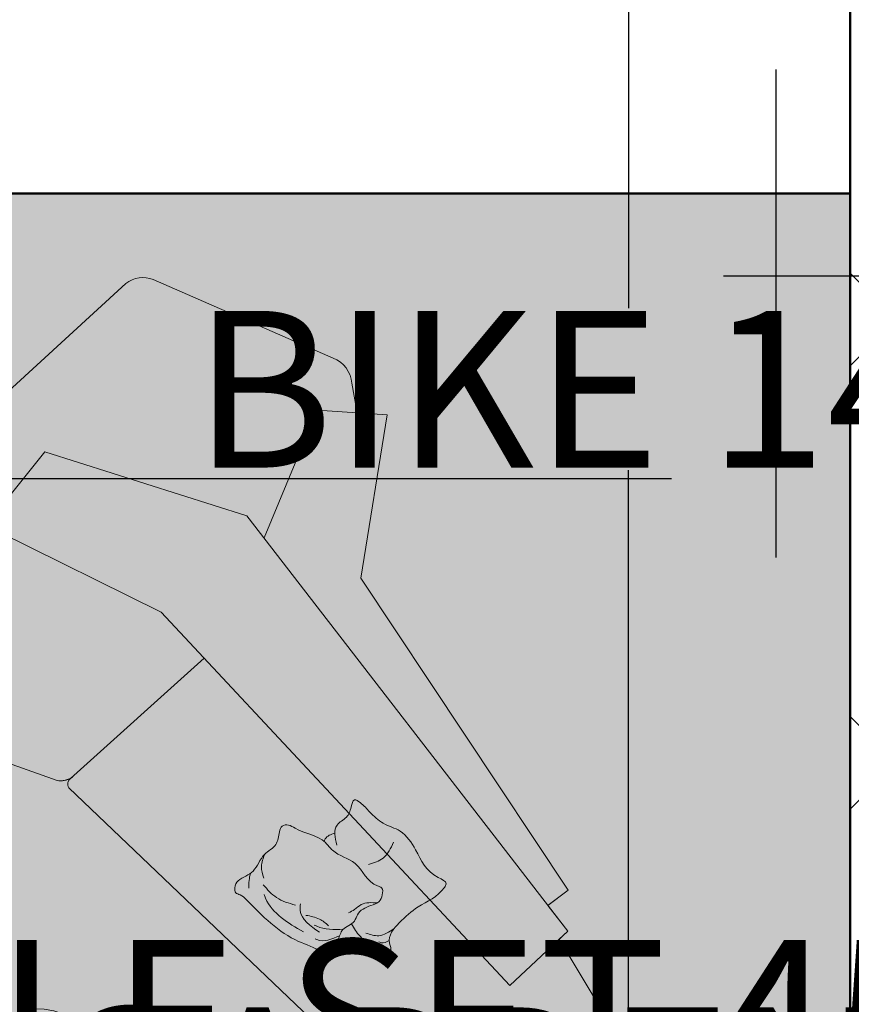
# Model space of a CAD drawing. Units: inches. Extents: x -466983 to 1020, y 324 to 318697.
# Tile 18 of 97: x 782 to 814, y 473 to 511. Entities that reach past the tile are written whole.
import ezdxf

# ---------------------------------------------------------------- set-up
doc = ezdxf.new("R2010")
doc.units = ezdxf.units.IN
doc.header["$MEASUREMENT"] = 0
for name, color, linetype, lineweight in [('A-ANNO-DIMS', 2, 'Continuous', 18), ('A-FLOR-PATT', 252, 'Continuous', 13), ('A-FURN', 8, 'Continuous', 18), ('A-WALL', 7, 'Continuous', 50)]:
    doc.layers.add(name, color=color, linetype=linetype, lineweight=lineweight)
doc.layers.add('K-Hatch', color=7, linetype='Continuous')
doc.styles.get("Standard").update_dxf_attribs({"font": 'arial.ttf'})
doc.dimstyles.get("Standard").update_dxf_attribs({"dimtxt": 6, "dimasz": 4, "dimexe": 3, "dimexo": 3, "dimgap": 0.09, "dimtad": 0, "dimtih": 1, "dimtoh": 1, "dimdec": 1, "dimzin": 0, "dimdsep": 46, "dimlunit": 3, "dimtxsty": 'Standard', "dimcen": 0.09, "dimadec": 0, "dimazin": 0, "dimtfac": 1, "dimtdec": 1, "dimtofl": 0, "dimtmove": 0, "dimatfit": 3, "dimfxl": 1, "dimtolj": 1, "dimtzin": 0, "dimarcsym": 0})

# ---------------------------------------------------------------- blocks, each defined once
blk = doc.blocks.new('CBV_08')
at = {"layer": 'K-Hatch'}
h = blk.add_hatch(color=256, dxfattribs=at)
h.dxf.hatch_style = 1
h.set_gradient(color1=(254, 240, 205), color2=(128, 128, 128), name='INVSPHERICAL')
edge = h.paths.add_edge_path()
edge.add_line((-64.8, 606.5), (-20.8, 613.5))
edge.add_line((-20.8, 613.5), (24.3, 618.7))
edge.add_line((24.3, 618.7), (72.9, 622.4))
edge.add_line((72.9, 622.4), (121.2, 624.4))
edge.add_line((121.2, 624.4), (138, 624.4))
edge.add_spline(control_points=[(138, 624.4), (115.4, 642), (92.5, 659.2), (69.5, 676.1)], knot_values=[4, 4, 4, 4, 4.295361, 4.295361, 4.295361, 4.295361], degree=3, periodic=0)
edge.add_spline(control_points=[(69.5, 676.1), (30.7, 704.6), (-11, 728.2), (-55.3, 747.2)], knot_values=[3, 3, 3, 3, 4, 4, 4, 4], degree=3, periodic=0)
edge.add_spline(control_points=[(-55.3, 747.2), (-74.8, 755.6), (-96, 763.3), (-117, 767)], knot_values=[2, 2, 2, 2, 3, 3, 3, 3], degree=3, periodic=0)
edge.add_spline(control_points=[(-117, 767), (-129.2, 769.1), (-142.6, 773.4), (-154.9, 773.6)], knot_values=[1, 1, 1, 1, 2, 2, 2, 2], degree=3, periodic=0)
edge.add_spline(control_points=[(-154.9, 773.6), (-167.5, 773.8), (-180, 774.1), (-192.6, 774.3)], knot_values=[0, 0, 0, 0, 1, 1, 1, 1], degree=3, periodic=0)
edge.add_spline(control_points=[(-192.6, 774.3), (-216.8, 770.8), (-242.2, 768.1), (-264.6, 757.4)], knot_values=[36, 36, 36, 36, 37, 37, 37, 37], degree=3, periodic=0)
edge.add_spline(control_points=[(-264.6, 757.4), (-290.4, 745.1), (-313.9, 731.3), (-338.2, 716.3)], knot_values=[35, 35, 35, 35, 36, 36, 36, 36], degree=3, periodic=0)
edge.add_spline(control_points=[(-338.2, 716.3), (-348, 710.3), (-356.8, 702.3), (-365.9, 695.4)], knot_values=[34, 34, 34, 34, 35, 35, 35, 35], degree=3, periodic=0)
edge.add_spline(control_points=[(-365.9, 695.4), (-373.7, 689.5), (-381.9, 684), (-389, 677.3)], knot_values=[33, 33, 33, 33, 34, 34, 34, 34], degree=3, periodic=0)
edge.add_spline(control_points=[(-389, 677.3), (-406.7, 660.6), (-425.2, 644.6), (-441, 625.9)], knot_values=[32, 32, 32, 32, 33, 33, 33, 33], degree=3, periodic=0)
edge.add_spline(control_points=[(-441, 625.9), (-457.4, 606.6), (-473.1, 588.1), (-486.9, 566.8)], knot_values=[31, 31, 31, 31, 32, 32, 32, 32], degree=3, periodic=0)
edge.add_spline(control_points=[(-486.9, 566.8), (-500.9, 545.3), (-513.6, 524.6), (-525.3, 501.8)], knot_values=[30, 30, 30, 30, 31, 31, 31, 31], degree=3, periodic=0)
edge.add_spline(control_points=[(-525.3, 501.8), (-537.3, 478.5), (-547, 455.6), (-556.5, 431.1)], knot_values=[29, 29, 29, 29, 30, 30, 30, 30], degree=3, periodic=0)
edge.add_spline(control_points=[(-556.5, 431.1), (-560.1, 422), (-562.6, 413.9), (-564.7, 404.4)], knot_values=[28, 28, 28, 28, 29, 29, 29, 29], degree=3, periodic=0)
edge.add_spline(control_points=[(-564.7, 404.4), (-567.4, 392.4), (-572.8, 378.6), (-573.3, 366.3)], knot_values=[27, 27, 27, 27, 28, 28, 28, 28], degree=3, periodic=0)
edge.add_spline(control_points=[(-573.3, 366.3), (-574.1, 341.5), (-575.3, 317.8), (-572.6, 293.2)], knot_values=[26, 26, 26, 26, 27, 27, 27, 27], degree=3, periodic=0)
edge.add_spline(control_points=[(-572.6, 293.2), (-569.8, 268.3), (-564.7, 244.8), (-559.2, 220.4)], knot_values=[25, 25, 25, 25, 26, 26, 26, 26], degree=3, periodic=0)
edge.add_spline(control_points=[(-559.2, 220.4), (-554.1, 197.5), (-542.3, 175), (-531.2, 154.5)], knot_values=[24, 24, 24, 24, 25, 25, 25, 25], degree=3, periodic=0)
edge.add_spline(control_points=[(-531.2, 154.5), (-519.4, 132.5), (-505, 113.3), (-490.3, 93.1)], knot_values=[23, 23, 23, 23, 24, 24, 24, 24], degree=3, periodic=0)
edge.add_spline(control_points=[(-490.3, 93.1), (-483.4, 83.5), (-474, 75.1), (-466, 66.4)], knot_values=[22, 22, 22, 22, 23, 23, 23, 23], degree=3, periodic=0)
edge.add_spline(control_points=[(-466, 66.4), (-459.7, 59.5), (-453.6, 52.4), (-446.7, 46)], knot_values=[21, 21, 21, 21, 22, 22, 22, 22], degree=3, periodic=0)
edge.add_spline(control_points=[(-446.7, 46), (-428.9, 29.8), (-411.7, 12.8), (-392.8, -2.2)], knot_values=[20, 20, 20, 20, 21, 21, 21, 21], degree=3, periodic=0)
edge.add_spline(control_points=[(-392.8, -2.2), (-354.9, -32.3), (-316.7, -63.5), (-274.7, -87.8)], knot_values=[19, 19, 19, 19, 20, 20, 20, 20], degree=3, periodic=0)
edge.add_spline(control_points=[(-274.7, -87.8), (-235, -110.9), (-195.1, -133.6), (-153.3, -152.9)], knot_values=[18.058389, 18.058389, 18.058389, 18.058389, 19, 19, 19, 19], degree=3, periodic=0)
edge.add_arc((49.9, -261.3), 230.3, 65.0387, 151.9024, ccw=False)
edge.add_arc((-129.3, -568), 584.8, 31.4853, 61.8022, ccw=False)
edge.add_spline(control_points=[(369.5, -262.5), (382.1, -256.3), (394.4, -248.9), (404.8, -240.3)], knot_values=[14, 14, 14, 14, 14.639139, 14.639139, 14.639139, 14.639139], degree=3, periodic=0)
edge.add_spline(control_points=[(404.8, -240.3), (441.3, -209.9), (479.6, -177), (505.1, -136.3)], knot_values=[13, 13, 13, 13, 14, 14, 14, 14], degree=3, periodic=0)
edge.add_spline(control_points=[(505.1, -136.3), (530.8, -95.3), (553.2, -52.4), (563.4, -4.8)], knot_values=[12, 12, 12, 12, 13, 13, 13, 13], degree=3, periodic=0)
edge.add_spline(control_points=[(563.4, -4.8), (565.9, 6.8), (569.9, 18.9), (570.9, 30.6)], knot_values=[11, 11, 11, 11, 12, 12, 12, 12], degree=3, periodic=0)
edge.add_spline(control_points=[(570.9, 30.6), (572, 44.6), (573.1, 58.6), (574.2, 72.5)], knot_values=[10, 10, 10, 10, 11, 11, 11, 11], degree=3, periodic=0)
edge.add_spline(control_points=[(574.2, 72.5), (575.1, 84.1), (571.6, 97.4), (570.3, 109)], knot_values=[9, 9, 9, 9, 10, 10, 10, 10], degree=3, periodic=0)
edge.add_spline(control_points=[(570.3, 109), (569.1, 120.8), (562.9, 133.2), (559.3, 144.5)], knot_values=[8, 8, 8, 8, 9, 9, 9, 9], degree=3, periodic=0)
edge.add_spline(control_points=[(559.3, 144.5), (552.8, 164.6), (542, 184.7), (531.4, 203)], knot_values=[7, 7, 7, 7, 8, 8, 8, 8], degree=3, periodic=0)
edge.add_spline(control_points=[(531.4, 203), (517.9, 226.2), (504.2, 248.2), (488.9, 270.1)], knot_values=[6, 6, 6, 6, 7, 7, 7, 7], degree=3, periodic=0)
edge.add_spline(control_points=[(488.9, 270.1), (469.9, 297.6), (449.2, 323.8), (427.6, 349.1)], knot_values=[5.661323, 5.661323, 5.661323, 5.661323, 6, 6, 6, 6], degree=3, periodic=0)
edge.add_line((427.6, 349.1), (424, 340.6))
edge.add_line((424, 340.6), (412.8, 320.4))
edge.add_line((412.8, 320.4), (399.8, 302.2))
edge.add_line((399.8, 302.2), (384.1, 283.9))
edge.add_line((384.1, 283.9), (364.2, 265.4))
edge.add_line((364.2, 265.4), (338.9, 246.4))
edge.add_line((338.9, 246.4), (310.9, 228.8))
edge.add_line((310.9, 228.8), (283, 214))
edge.add_line((283, 214), (254.8, 200.7))
edge.add_line((254.8, 200.7), (225.6, 187.8))
edge.add_line((225.6, 187.8), (191.9, 174.7))
edge.add_line((191.9, 174.7), (149.8, 160.6))
edge.add_line((149.8, 160.6), (105.2, 147.1))
edge.add_line((105.2, 147.1), (63.8, 135.5))
edge.add_line((63.8, 135.5), (25.5, 126.4))
edge.add_line((25.5, 126.4), (-10.1, 120.3))
edge.add_line((-10.1, 120.3), (-42.7, 117))
edge.add_line((-42.7, 117), (-72.3, 116.4))
edge.add_line((-72.3, 116.4), (-101, 119.4))
edge.add_line((-101, 119.4), (-131.2, 126.4))
edge.add_line((-131.2, 126.4), (-161, 137.6))
edge.add_line((-161, 137.6), (-188.5, 153.1))
edge.add_line((-188.5, 153.1), (-212.6, 173.8))
edge.add_line((-212.6, 173.8), (-232.4, 200.6))
edge.add_line((-232.4, 200.6), (-247.5, 230.4))
edge.add_line((-247.5, 230.4), (-258, 260.2))
edge.add_line((-258, 260.2), (-265.5, 290.4))
edge.add_line((-265.5, 290.4), (-271.7, 321.1))
edge.add_line((-271.7, 321.1), (-275.7, 353.5))
edge.add_line((-275.7, 353.5), (-276.1, 388.5))
edge.add_line((-276.1, 388.5), (-273.5, 421.6))
edge.add_line((-273.5, 421.6), (-268.6, 448.2))
edge.add_line((-268.6, 448.2), (-261.6, 470.9))
edge.add_line((-261.6, 470.9), (-253.2, 492.6))
edge.add_line((-253.2, 492.6), (-243.7, 512.2))
edge.add_line((-243.7, 512.2), (-233.7, 528.6))
edge.add_line((-233.7, 528.6), (-222.4, 543.2))
edge.add_line((-222.4, 543.2), (-208.8, 557))
edge.add_line((-208.8, 557), (-193, 569.1))
edge.add_line((-193, 569.1), (-174.9, 578.6))
edge.add_line((-174.9, 578.6), (-149, 587.3))
edge.add_line((-149, 587.3), (-109.9, 597.2))
edge.add_line((-109.9, 597.2), (-64.8, 606.5))
edge = h.paths.add_edge_path()
edge.add_spline(control_points=[(370.8, -764.2), (495.7, -715.3), (556.2, -553.3), (490.4, -435.8)], knot_values=[8, 8, 8, 8, 9, 9, 9, 9], degree=3, periodic=0)
edge.add_spline(control_points=[(490.4, -435.8), (456.6, -375.3), (415.1, -316.6), (369.5, -262.5)], knot_values=[7.311196, 7.311196, 7.311196, 7.311196, 8, 8, 8, 8], degree=3, periodic=0)
edge.add_spline(control_points=[(369.5, -262.5), (362.3, -266), (355, -269.1), (347.9, -271.7)], knot_values=[14.639139, 14.639139, 14.639139, 14.639139, 15, 15, 15, 15], degree=3, periodic=0)
edge.add_spline(control_points=[(347.9, -271.7), (326, -279.9), (303.4, -287.9), (279.6, -286.9)], knot_values=[15, 15, 15, 15, 16, 16, 16, 16], degree=3, periodic=0)
edge.add_spline(control_points=[(279.6, -286.9), (229.3, -284.8), (181, -274.1), (132.3, -261.7)], knot_values=[16, 16, 16, 16, 17, 17, 17, 17], degree=3, periodic=0)
edge.add_spline(control_points=[(132.3, -261.7), (36, -237.2), (-55, -196.9), (-145.5, -156.4)], knot_values=[17, 17, 17, 17, 18, 18, 18, 18], degree=3, periodic=0)
edge.add_spline(control_points=[(-145.5, -156.4), (-148.1, -155.2), (-150.7, -154.1), (-153.3, -152.9)], knot_values=[18, 18, 18, 18, 18.058389, 18.058389, 18.058389, 18.058389], degree=3, periodic=0)
edge.add_spline(control_points=[(-274.7, -87.8), (-235, -110.9), (-195.1, -133.6), (-153.3, -152.9)], knot_values=[18.058389, 18.058389, 18.058389, 18.058389, 19, 19, 19, 19], degree=3, periodic=0)
edge.add_spline(control_points=[(-153.3, -152.9), (-166, -171.6), (-175.5, -191.9), (-179.2, -212.7)], knot_values=[4, 4, 4, 4, 4.452929, 4.452929, 4.452929, 4.452929], degree=3, periodic=0)
edge.add_spline(control_points=[(-179.2, -212.7), (-197.4, -316.3), (-177.2, -425), (-133.8, -520.2)], knot_values=[3, 3, 3, 3, 4, 4, 4, 4], degree=3, periodic=0)
edge.add_spline(control_points=[(-133.8, -520.2), (-113.8, -564.2), (-89.7, -609.8), (-55.6, -644.7)], knot_values=[2, 2, 2, 2, 3, 3, 3, 3], degree=3, periodic=0)
edge.add_spline(control_points=[(-55.6, -644.7), (-21, -680), (24.1, -705.5), (69.8, -723.3)], knot_values=[1, 1, 1, 1, 2, 2, 2, 2], degree=3, periodic=0)
edge.add_spline(control_points=[(69.8, -723.3), (165.7, -760.7), (268.3, -790.7), (370.8, -764.2)], knot_values=[0, 0, 0, 0, 1, 1, 1, 1], degree=3, periodic=0)
h = blk.add_hatch(color=256, dxfattribs=at)
h.dxf.hatch_style = 1
h.set_gradient(color1=(237, 238, 153), color2=(128, 128, 128), name='INVSPHERICAL')
h.paths.add_polyline_path([(138, 624.4), (121.2, 624.4), (72.9, 622.4), (24.3, 618.7), (-20.8, 613.5), (-64.8, 606.5), (-109.9, 597.2), (-149, 587.3), (-174.9, 578.6), (-193, 569.1), (-208.8, 557), (-222.4, 543.2), (-233.7, 528.6), (-243.7, 512.2), (-253.2, 492.6), (-261.6, 470.9), (-268.6, 448.2), (-273.5, 421.6), (-276.1, 388.5), (-275.7, 353.5), (-271.7, 321.1), (-265.5, 290.4), (-258, 260.2), (-247.5, 230.4), (-232.4, 200.6), (-212.6, 173.8), (-188.5, 153.1), (-161, 137.6), (-131.2, 126.4), (-101, 119.4), (-72.3, 116.4), (-42.7, 117), (-10.1, 120.3), (25.5, 126.4), (63.8, 135.5), (105.2, 147.1), (149.8, 160.6), (191.9, 174.7), (225.6, 187.8), (254.8, 200.7), (283, 214), (310.9, 228.8), (338.9, 246.4), (364.2, 265.4), (384.1, 283.9), (399.8, 302.2), (412.8, 320.4), (424, 340.6), (427.6, 349.1, 0.092765)])
h.paths.add_polyline_path([(388.8, 558), (367.1, 577.3), (341.1, 593.1), (309.7, 604.8), (275.6, 613.2), (241.4, 619.1), (205.2, 622.8), (165.2, 624.5), (138, 624.4, -0.092765), (427.6, 349.1), (434.3, 364.7), (441.6, 390.8), (443.8, 416.8), (441.1, 445), (433.5, 477.6), (421.8, 509.5), (406.9, 535.9)])
edge = h.paths.add_edge_path()
edge.add_arc((49.9, -261.3), 230.3, 65.0387, 151.9024)
edge.add_spline(control_points=[(-153.3, -152.9), (-150.7, -154.1), (-148.1, -155.2), (-145.5, -156.4)], knot_values=[18, 18, 18, 18, 18.058389, 18.058389, 18.058389, 18.058389], degree=3, periodic=0)
edge.add_spline(control_points=[(-145.5, -156.4), (-55, -196.9), (36, -237.2), (132.3, -261.7)], knot_values=[17, 17, 17, 17, 18, 18, 18, 18], degree=3, periodic=0)
edge.add_spline(control_points=[(132.3, -261.7), (181, -274.1), (229.3, -284.8), (279.6, -286.9)], knot_values=[16, 16, 16, 16, 17, 17, 17, 17], degree=3, periodic=0)
edge.add_spline(control_points=[(279.6, -286.9), (303.4, -287.9), (326, -279.9), (347.9, -271.7)], knot_values=[15, 15, 15, 15, 16, 16, 16, 16], degree=3, periodic=0)
edge.add_spline(control_points=[(347.9, -271.7), (355, -269.1), (362.3, -266), (369.5, -262.5)], knot_values=[14.639139, 14.639139, 14.639139, 14.639139, 15, 15, 15, 15], degree=3, periodic=0)
edge.add_arc((-129.3, -568), 584.8, 31.4853, 61.8022)
edge = h.paths.add_edge_path()
edge.add_spline(control_points=[(490.4, -435.8), (456.6, -375.3), (415.1, -316.6), (369.5, -262.5)], knot_values=[7.311196, 7.311196, 7.311196, 7.311196, 8, 8, 8, 8], degree=3, periodic=0)
edge.add_spline(control_points=[(369.5, -262.5), (362.3, -266), (355, -269.1), (347.9, -271.7)], knot_values=[14.639139, 14.639139, 14.639139, 14.639139, 15, 15, 15, 15], degree=3, periodic=0)
edge.add_spline(control_points=[(347.9, -271.7), (326, -279.9), (303.4, -287.9), (279.6, -286.9)], knot_values=[15, 15, 15, 15, 16, 16, 16, 16], degree=3, periodic=0)
edge.add_spline(control_points=[(279.6, -286.9), (229.3, -284.8), (181, -274.1), (132.3, -261.7)], knot_values=[16, 16, 16, 16, 17, 17, 17, 17], degree=3, periodic=0)
edge.add_spline(control_points=[(132.3, -261.7), (36, -237.2), (-55, -196.9), (-145.5, -156.4)], knot_values=[17, 17, 17, 17, 18, 18, 18, 18], degree=3, periodic=0)
edge.add_spline(control_points=[(-145.5, -156.4), (-148.1, -155.2), (-150.7, -154.1), (-153.3, -152.9)], knot_values=[18, 18, 18, 18, 18.058389, 18.058389, 18.058389, 18.058389], degree=3, periodic=0)
edge.add_spline(control_points=[(-274.7, -87.8), (-235, -110.9), (-195.1, -133.6), (-153.3, -152.9)], knot_values=[18.058389, 18.058389, 18.058389, 18.058389, 19, 19, 19, 19], degree=3, periodic=0)
edge.add_spline(control_points=[(-153.3, -152.9), (-166, -171.6), (-175.5, -191.9), (-179.2, -212.7)], knot_values=[4, 4, 4, 4, 4.452929, 4.452929, 4.452929, 4.452929], degree=3, periodic=0)
edge.add_spline(control_points=[(-179.2, -212.7), (-197.4, -316.3), (-177.2, -425), (-133.8, -520.2)], knot_values=[3, 3, 3, 3, 4, 4, 4, 4], degree=3, periodic=0)
edge.add_spline(control_points=[(-133.8, -520.2), (-113.8, -564.2), (-89.7, -609.8), (-55.6, -644.7)], knot_values=[2, 2, 2, 2, 3, 3, 3, 3], degree=3, periodic=0)
edge.add_spline(control_points=[(-55.6, -644.7), (-21, -680), (24.1, -705.5), (69.8, -723.3)], knot_values=[1, 1, 1, 1, 2, 2, 2, 2], degree=3, periodic=0)
edge.add_spline(control_points=[(69.8, -723.3), (165.7, -760.7), (268.3, -790.7), (370.8, -764.2)], knot_values=[0, 0, 0, 0, 1, 1, 1, 1], degree=3, periodic=0)
edge.add_spline(control_points=[(370.8, -764.2), (495.7, -715.3), (556.2, -553.3), (490.4, -435.8)], knot_values=[8, 8, 8, 8, 9, 9, 9, 9], degree=3, periodic=0)
for points in [[(24.3, 618.7), (-20.8, 613.5)], [(72.9, 622.4), (24.3, 618.7)], [(121.2, 624.4), (72.9, 622.4)], [(121.2, 624.4), (72.9, 622.4)], [(165.2, 624.5), (121.2, 624.4)], [(205.2, 622.8), (165.2, 624.5)], [(241.4, 619.1), (205.2, 622.8)], [(275.6, 613.2), (241.4, 619.1)], [(-149, 587.3), (-174.9, 578.6)], [(-109.9, 597.2), (-149, 587.3)], [(-64.8, 606.5), (-109.9, 597.2)], [(-20.8, 613.5), (-64.8, 606.5)], [(309.7, 604.8), (275.6, 613.2)], [(341.1, 593.1), (309.7, 604.8)], [(367.1, 577.3), (341.1, 593.1)], [(-208.8, 557), (-222.4, 543.2)], [(-193, 569.1), (-208.8, 557)], [(-174.9, 578.6), (-193, 569.1)], [(388.8, 558), (367.1, 577.3)], [(406.9, 535.9), (388.8, 558)], [(-233.7, 528.6), (-243.7, 512.2)], [(-222.4, 543.2), (-233.7, 528.6)], [(421.8, 509.5), (406.9, 535.9)], [(-253.2, 492.6), (-261.6, 470.9)], [(-243.7, 512.2), (-253.2, 492.6)], [(433.5, 477.6), (421.8, 509.5)], [(-268.6, 448.2), (-273.5, 421.6)], [(-261.6, 470.9), (-268.6, 448.2)], [(441.1, 445), (433.5, 477.6)], [(-273.5, 421.6), (-276.1, 388.5)], [(443.8, 416.8), (441.1, 445)], [(441.6, 390.8), (443.8, 416.8)], [(-276.1, 388.5), (-275.7, 353.5)], [(434.3, 364.7), (441.6, 390.8)], [(-275.7, 353.5), (-271.7, 321.1)], [(424, 340.6), (434.3, 364.7)], [(-271.7, 321.1), (-265.5, 290.4)], [(399.8, 302.2), (412.8, 320.4)], [(412.8, 320.4), (424, 340.6)], [(-265.5, 290.4), (-258, 260.2)], [(364.2, 265.4), (384.1, 283.9)], [(384.1, 283.9), (399.8, 302.2)], [(-258, 260.2), (-247.5, 230.4)], [(310.9, 228.8), (338.9, 246.4)], [(338.9, 246.4), (364.2, 265.4)], [(-247.5, 230.4), (-232.4, 200.6)], [(254.8, 200.7), (283, 214)], [(254.8, 200.7), (283, 214)], [(283, 214), (310.9, 228.8)], [(-232.4, 200.6), (-212.6, 173.8)], [(-212.6, 173.8), (-188.5, 153.1)], [(149.8, 160.6), (191.9, 174.7)], [(149.8, 160.6), (191.9, 174.7)], [(191.9, 174.7), (225.6, 187.8)], [(225.6, 187.8), (254.8, 200.7)], [(227.5, 188.7), (226.1, 188.1)], [(-188.5, 153.1), (-161, 137.6)], [(-161, 137.6), (-131.2, 126.4)], [(63.8, 135.5), (105.2, 147.1)], [(105.2, 147.1), (149.8, 160.6)], [(-131.2, 126.4), (-101, 119.4)], [(-101, 119.4), (-72.3, 116.4)], [(-72.3, 116.4), (-42.7, 117)], [(-42.7, 117), (-10.1, 120.3)], [(-10.1, 120.3), (25.5, 126.4)], [(25.5, 126.4), (63.8, 135.5)]]:
    blk.add_lwpolyline(points)
at = {"ltscale": 150}
for centre, radius, start, end in [((-452.8, -286.9), 1086.1, 35.8442, 57.0436), ((49.9, -261.3), 230.3, 65.0387, 151.9024), ((-129.3, -568), 584.8, 31.4853, 61.8022)]:
    blk.add_arc(centre, radius, start, end, dxfattribs=at)
for points, knots in [([(427.6, 349.1), (449.2, 323.8), (469.9, 297.6), (488.9, 270.1), (504.2, 248.2), (517.9, 226.2), (531.4, 203), (542, 184.7), (552.8, 164.6), (559.3, 144.5), (562.9, 133.2), (569.1, 120.8), (570.3, 109), (571.6, 97.4), (575.1, 84.1), (574.2, 72.5), (573.1, 58.6), (572, 44.6), (570.9, 30.6), (569.9, 18.9), (565.9, 6.8), (563.4, -4.8), (553.2, -52.4), (530.8, -95.3), (505.1, -136.3), (479.6, -177), (441.3, -209.9), (404.8, -240.3), (388.6, -253.7), (367.6, -264.4), (347.9, -271.7), (326, -279.9), (303.4, -287.9), (279.6, -286.9), (229.3, -284.8), (181, -274.1), (132.3, -261.7), (36, -237.2), (-55, -196.9), (-145.5, -156.4), (-190.2, -136.4), (-232.5, -112.4), (-274.7, -87.8), (-316.7, -63.5), (-354.9, -32.3), (-392.8, -2.2), (-411.7, 12.8), (-428.9, 29.8), (-446.7, 46), (-453.6, 52.4), (-459.7, 59.5), (-466, 66.4), (-474, 75.1), (-483.4, 83.5), (-490.3, 93.1), (-505, 113.3), (-519.4, 132.5), (-531.2, 154.5), (-542.3, 175), (-554.1, 197.5), (-559.2, 220.4), (-564.7, 244.8), (-569.8, 268.3), (-572.6, 293.2), (-575.3, 317.8), (-574.1, 341.5), (-573.3, 366.3), (-572.8, 378.6), (-567.4, 392.4), (-564.7, 404.4), (-562.6, 413.9), (-560.1, 422), (-556.5, 431.1), (-547, 455.6), (-537.3, 478.5), (-525.3, 501.8), (-513.6, 524.6), (-500.9, 545.3), (-486.9, 566.8), (-473.1, 588.1), (-457.4, 606.6), (-441, 625.9), (-425.2, 644.6), (-406.7, 660.6), (-389, 677.3), (-381.9, 684), (-373.7, 689.5), (-365.9, 695.4), (-356.8, 702.3), (-348, 710.3), (-338.2, 716.3), (-313.9, 731.3), (-290.4, 745.1), (-264.6, 757.4), (-242.2, 768.1), (-216.8, 770.8), (-192.6, 774.3)], [5.661323, 5.661323, 5.661323, 5.661323, 6, 6, 6, 7, 7, 7, 8, 8, 8, 9, 9, 9, 10, 10, 10, 11, 11, 11, 12, 12, 12, 13, 13, 13, 14, 14, 14, 15, 15, 15, 16, 16, 16, 17, 17, 17, 18, 18, 18, 19, 19, 19, 20, 20, 20, 21, 21, 21, 22, 22, 22, 23, 23, 23, 24, 24, 24, 25, 25, 25, 26, 26, 26, 27, 27, 27, 28, 28, 28, 29, 29, 29, 30, 30, 30, 31, 31, 31, 32, 32, 32, 33, 33, 33, 34, 34, 34, 35, 35, 35, 36, 36, 36, 37, 37, 37, 37]), ([(-192.6, 774.3), (-180, 774.1), (-167.5, 773.8), (-154.9, 773.6), (-142.6, 773.4), (-129.2, 769.1), (-117, 767), (-96, 763.3), (-74.8, 755.6), (-55.3, 747.2), (-11, 728.2), (30.7, 704.6), (69.5, 676.1), (92.5, 659.2), (115.4, 642), (138, 624.4)], [0, 0, 0, 0, 1, 1, 1, 2, 2, 2, 3, 3, 3, 4, 4, 4, 4.295361, 4.295361, 4.295361, 4.295361]), ([(370.8, -764.2), (268.3, -790.7), (165.7, -760.7), (69.8, -723.3), (24.1, -705.5), (-21, -680), (-55.6, -644.7), (-89.7, -609.8), (-113.8, -564.2), (-133.8, -520.2), (-177.2, -425), (-197.4, -316.3), (-179.2, -212.7), (-175.5, -191.9), (-166, -171.6), (-153.3, -152.9)], [0, 0, 0, 0, 1, 1, 1, 2, 2, 2, 3, 3, 3, 4, 4, 4, 4.452929, 4.452929, 4.452929, 4.452929]), ([(369.5, -262.5), (415.1, -316.6), (456.6, -375.3), (490.4, -435.8), (556.2, -553.3), (495.7, -715.3), (370.8, -764.2)], [7.311196, 7.311196, 7.311196, 7.311196, 8, 8, 8, 9, 9, 9, 9])]:
    blk.add_open_spline(points, degree=3, knots=knots)
blk = doc.blocks.new('CBV_05')
at = {"layer": 'K-Hatch'}
h = blk.add_hatch(color=256, dxfattribs=at)
h.dxf.hatch_style = 1
h.paths.add_polyline_path([(614, 437), (1251.4, 62.5), (1198.3, -263.2), (564.8, -9.8), (344.4, -5.5), (343.7, -629.7, 0.159768), (369.9, -672.6), (1020.5, -1025.6, 0.317347), (1135.5, -1017.7), (1739.5, -492.7, 0.378101), (1761.2, -362.2), (1507.4, -70.4, -0.119239), (1492.6, -25.8), (1499.5, 665.1, 0.256804), (1446.2, 745.4), (822.7, 1028.7, 0.297137), (714, 1018.3), (625, 963.6), (549.5, 1037.1), (186.8, 587.5), (-1106.2, 397.7), (-1098.6, 311.5), (-1098.4, 310.2)])
h.paths.add_polyline_path([(344.4, -5.5), (-1216.9, 24.6), (-1212.3, 260), (-1718.1, 162.7, 0.51466), (-1765.1, 50), (-1478.1, -479.5, 0.244482), (-1398.8, -526.6), (323.6, -658.2, 0.453292), (343.1, -629.8, 0.006511), (343.7, -631.8)])
h = blk.add_hatch(color=256, dxfattribs=at)
h.dxf.hatch_style = 1
h.paths.add_polyline_path([(614, 437), (-1211.5, 301.9), (-1212.3, 260), (-1216.9, 24.6), (564.8, -9.8), (1198.3, -263.2), (1251.4, 62.5)])
for p, q in [((186.8, 587.5), (549.5, 1037.1)), ((725.2, 866.1), (549.5, 1037.1)), ((517.5, 431), (725.2, 866.1)), ((-1106.2, 397.7), (186.8, 587.5)), ((-1211.5, 301.9), (614, 437)), ((614, 437), (1251.4, 62.5)), ((-1106.2, 397.7), (-1098.6, 311.5)), ((-1211.5, 301.9), (-1216.9, 24.6)), ((1251.4, 62.5), (1198.3, -263.2)), ((-1216.9, 24.6), (564.8, -9.8)), ((564.8, -9.8), (1198.3, -263.2))]:
    blk.add_line(p, q)
blk.add_lwpolyline([(1761.2, -362.2, -0.378101), (1739.5, -492.7), (1135.5, -1017.7, -0.317347), (1020.5, -1025.6), (369.9, -672.6, -0.159481), (343.2, -630.1, -0.449095), (323.6, -658.2), (-1398.8, -526.6, -0.244482), (-1478.1, -479.5), (-1765.1, 50, -0.51466), (-1718.1, 162.7), (-1212.3, 260), (-1211.5, 301.9), (-1098.4, 310.2), (-1106.2, 397.7), (186.8, 587.5), (549.5, 1037.1), (625, 963.6), (714, 1018.3, -0.297137), (822.7, 1028.7), (1446.2, 745.4, -0.256804), (1499.5, 665.1), (1492.6, -25.8, 0.119239), (1507.4, -70.4)], format="xyb", close=True)
for points in [[(369.9, -672.6), (1020.5, -1025.6, 0.317347), (1135.5, -1017.7), (1739.5, -492.7, 0.378101), (1761.2, -362.2), (1507.4, -70.4, -0.119239), (1492.6, -25.8), (1499.5, 665.1, 0.256804), (1446.2, 745.4), (822.7, 1028.7, 0.297137), (714, 1018.3), (625, 963.6)], [(-1212.3, 260), (-1718.1, 162.7, 0.51466), (-1765.1, 50), (-1478.1, -479.5, 0.244482), (-1398.8, -526.6), (323.6, -658.2)]]:
    blk.add_lwpolyline(points, format="xyb")
blk.add_lwpolyline([(344.4, -5.5), (343.7, -632.6)])
for centre, radius, start, end in [((320.9, -635.5), 22.9, 276.7908, 7.9615), ((422.2, -611.1), 80.7, 188.9571, 229.6497)]:
    blk.add_arc(centre, radius, start, end)
blk = doc.blocks.new('CBV_02')
for points, knots in [([(-91.4, -131.3), (-106.3, -141.3), (-144.4, -166.7), (-198.1, -169.3), (-239.8, -177.4), (-263.2, -156.4), (-220.4, -122.4), (-241.1, -51.6), (-276.5, 31.5), (-327.5, 83.5), (-334.1, 145.3), (-254.2, 139), (-199.8, 191.5), (-115.5, 242.2), (-44.1, 228.2), (13.9, 247.4), (48.9, 263.5), (90.2, 270.4), (80.3, 230.8), (77.5, 197.5), (114.6, 151.6), (88, 117.5), (71.5, 96.3)], [0, 0, 0, 0, 52.878976, 135.54457, 156.895053, 178.454765, 205.017242, 283.653969, 369.581717, 483.880697, 497.901213, 533.111935, 657.57549, 742.691795, 807.096717, 868.633311, 916.15584, 937.624163, 964.928306, 1003.93421, 1046.712597, 1116.246585, 1116.246585, 1116.246585, 1116.246585]), ([(-103.4, 189.4), (-103.5, 166.1), (-103.8, 123.2), (-72.3, 94.8), (-58, 81.8)], [0, 0, 0, 0, 66.320843, 121.78475, 121.78475, 121.78475, 121.78475]), ([(95.2, 131.1), (105.5, 121.2), (118.3, 108.9), (117.4, 92.3), (117.3, 89.1)], [0, 0, 0, 0, 39.264535, 48.815694, 48.815694, 48.815694, 48.815694]), ([(-146.1, 6), (-148.1, -3), (-149.3, -22.5), (-119, -49.5), (-92.3, -81.4), (-102.2, -127.6), (-64.2, -156.5), (-75.8, -196.4), (-68.5, -226.7), (-89.3, -248.7), (-66.3, -271), (-19, -258.2), (97, -276), (211.6, -235.3), (298.4, -201.8), (321.3, -207.8), (333.3, -187), (332.8, -160.3), (312.2, -137.2), (287.8, -99.3), (296.8, -44.1), (256.4, 5), (270.7, 44.3), (276.3, 77.1), (252.3, 90.7), (198.4, 81.4), (134.7, 104), (61.7, 61.2), (-24.3, 81.7), (-82.8, 19.8), (-138, 31.1), (-144, 15.2), (-146.1, 6)], [0, 0, 0, 0, 24.616915, 57.389552, 114.237533, 138.455284, 189.005997, 228.810774, 251.953092, 279.847444, 297.942972, 329.329631, 417.096019, 649.5591, 678.18061, 694.45516, 711.884356, 739.183211, 771.087794, 801.279315, 871.941271, 924.495086, 970.994857, 992.485443, 1014.330787, 1039.800329, 1156.628447, 1193.646246, 1284.736416, 1395.218734, 1410.912041, 1436.038203, 1436.038203, 1436.038203, 1436.038203]), ([(-142.3, -26.5), (-123.8, -33.7), (-95.7, -44.8), (-82, -80.3), (-71.1, -94.3), (-66.1, -100.7)], [0, 0, 0, 0, 56.119763, 85.047758, 109.497008, 109.497008, 109.497008, 109.497008]), ([(285.1, -38.6), (284.4, -54.2), (283, -84.1), (262.6, -105.9), (252.9, -116.4)], [0, 0, 0, 0, 45.245577, 86.676748, 86.676748, 86.676748, 86.676748]), ([(-233.2, -82.9), (-222.4, -100.8), (-203.2, -132.7), (-166.7, -136.8), (-150.7, -138.6)], [0, 0, 0, 0, 58.76228, 104.640212, 104.640212, 104.640212, 104.640212]), ([(-235.6, -127), (-229, -136.1), (-220.7, -147.8), (-207.6, -146.9), (-204.8, -146.7)], [0, 0, 0, 0, 30.082797, 38.252376, 38.252376, 38.252376, 38.252376]), ([(-73.5, -160.3), (-44.8, -174.7), (-13.3, -190.5), (21, -190), (24.2, -189.9)], [0, 0, 0, 0, 92.944368, 102.453901, 102.453901, 102.453901, 102.453901]), ([(-22.2, -170.9), (-9.3, -167.3), (19.5, -159.1), (48.5, -167.1), (64.6, -171.5)], [0, 0, 0, 0, 39.396451, 88.251181, 88.251181, 88.251181, 88.251181]), ([(-2.6, -204.8), (35.3, -198.3), (82, -190.4), (96.8, -150.5), (99.6, -143)], [0, 0, 0, 0, 101.132145, 124.532908, 124.532908, 124.532908, 124.532908]), ([(47.9, -227.8), (110.7, -221.9), (178.7, -215.5), (224.5, -170.7), (228, -167.3)], [0, 0, 0, 0, 176.788032, 191.44385, 191.44385, 191.44385, 191.44385]), ([(244.8, -137.9), (224.6, -146.9), (182.5, -165.9), (136.8, -158.5), (112.9, -154.6)], [0, 0, 0, 0, 64.853922, 135.586683, 135.586683, 135.586683, 135.586683]), ([(-72.1, -185.7), (-52.1, -208.3), (-30.7, -232.6), (-1.5, -232), (0.5, -232)], [0, 0, 0, 0, 81.161444, 87.060878, 87.060878, 87.060878, 87.060878])]:
    blk.add_open_spline(points, degree=3, knots=knots)
blk.add_open_spline([(285.5, -170.2), (292.7, -153.9), (299.9, -137.5), (302.1, -120.4)], degree=3)
blk = doc.blocks.new('Garden Sofa')
at = {"xscale": -0.0109740885734132, "yscale": 0.0109740885734132, "zscale": 0.0109740885734132}
for name, p, rotation in [('CBV_05', (2464.355, 846.083), 311.9356943688126), ('CBV_02', (2467.122, 840.412), 334.8587275215129), ('CBV_08', (2451.373, 829.781), 280.5267845499334)]:
    blk.add_blockref(name, p, dxfattribs=dict(at, rotation=rotation))
blk = doc.blocks.new('*D70')
at = {"layer": 'A-ANNO-DIMS', "color": 0, "lineweight": -2, "transparency": 16777216}
for p, q in [((689.806, 508.686), (689.806, 490.005)), ((810.968, 508.686), (810.968, 490.005)), ((693.806, 493.005), (744.53, 493.005)), ((806.968, 493.005), (756.244, 493.005))]:
    blk.add_line(p, q, dxfattribs=at)
at = {"layer": 'A-ANNO-DIMS', "color": 0, "transparency": 16777216}
for points in [[(693.806, 493.671), (693.806, 492.338), (689.806, 493.005)], [(806.968, 493.671), (806.968, 492.338), (810.968, 493.005)]]:
    blk.add_solid(points, dxfattribs=at)
at = {"layer": 'Defpoints', "color": 0, "transparency": 16777216}
for p in [(689.806, 511.686), (810.968, 511.686), (810.968, 493.005)]:
    blk.add_point(p, dxfattribs=at)
at = {"layer": 'A-ANNO-DIMS', "color": 0, "transparency": 16777216, "insert": (750.387, 493.005), "char_height": 6, "attachment_point": 5}
blk.add_mtext('\\A1;121', dxfattribs=at)
blk = doc.blocks.new('*D93')
at = {"layer": 'A-ANNO-DIMS', "color": 0, "lineweight": -2, "transparency": 16777216}
for p, q in [((808.966, 500.777), (818.266, 500.777)), ((815.266, 496.777), (815.266, 472.969)), ((815.266, 442.777), (815.266, 466.584)), ((808.966, 438.777), (818.266, 438.777))]:
    blk.add_line(p, q, dxfattribs=at)
at = {"layer": 'A-ANNO-DIMS', "color": 0, "transparency": 16777216}
for points in [[(814.599, 496.777), (815.933, 496.777), (815.266, 500.777)], [(814.599, 442.777), (815.933, 442.777), (815.266, 438.777)]]:
    blk.add_solid(points, dxfattribs=at)
at = {"layer": 'Defpoints', "color": 0, "transparency": 16777216}
for p in [(805.966, 500.777), (815.266, 500.777), (805.966, 438.777)]:
    blk.add_point(p, dxfattribs=at)
at = {"layer": 'A-ANNO-DIMS', "color": 0, "transparency": 16777216, "insert": (815.266, 469.777), "char_height": 6, "attachment_point": 5}
blk.add_mtext('\\A1;GARDEN SEAT 62', dxfattribs=at)
blk = doc.blocks.new('*D97')
at = {"layer": 'A-ANNO-DIMS', "color": 0, "lineweight": -2, "transparency": 16777216}
for p, q in [((823.929, 568.441), (802.329, 568.441)), ((805.329, 564.441), (805.329, 499.545)), ((805.329, 428.441), (805.329, 493.337)), ((823.929, 424.441), (802.329, 424.441))]:
    blk.add_line(p, q, dxfattribs=at)
at = {"layer": 'A-ANNO-DIMS', "color": 0, "transparency": 16777216}
for points in [[(804.662, 564.441), (805.996, 564.441), (805.329, 568.441)], [(804.662, 428.441), (805.996, 428.441), (805.329, 424.441)]]:
    blk.add_solid(points, dxfattribs=at)
at = {"layer": 'Defpoints', "color": 0, "transparency": 16777216}
for p in [(826.929, 568.441), (805.329, 424.441), (826.929, 424.441)]:
    blk.add_point(p, dxfattribs=at)
at = {"layer": 'A-ANNO-DIMS', "color": 0, "transparency": 16777216, "insert": (805.329, 496.441), "char_height": 6, "attachment_point": 5}
blk.add_mtext('\\A1;BIKE 144', dxfattribs=at)
blk = doc.blocks.new('*D113')
at = {"layer": 'A-ANNO-DIMS', "color": 0, "lineweight": -2, "transparency": 16777216}
for p, q in [((704.71, 504.652), (709.525, 509.413)), ((710.204, 504.46), (736.319, 478.049)), ((736.45, 472.553), (741.265, 477.314)), ((739.132, 475.204), (741.944, 472.36)), ((741.944, 472.36), (745.944, 472.36))]:
    blk.add_line(p, q, dxfattribs=at)
at = {"layer": 'A-ANNO-DIMS', "color": 0, "transparency": 16777216}
for points in [[(710.678, 504.928), (709.73, 503.991), (707.392, 507.304)], [(736.794, 478.517), (735.845, 477.58), (739.132, 475.204)]]:
    blk.add_solid(points, dxfattribs=at)
at = {"layer": 'Defpoints', "color": 0, "transparency": 16777216}
for p in [(702.577, 502.543), (739.132, 475.204), (734.317, 470.443)]:
    blk.add_point(p, dxfattribs=at)
at = {"layer": 'A-ANNO-DIMS', "color": 0, "transparency": 16777216, "insert": (783.502, 472.36), "char_height": 6, "attachment_point": 5}
blk.add_mtext('\\A1;TEA TABLE SET 45', dxfattribs=at)

msp = doc.modelspace()

# ---------------------------------------------------------------- hatches: boundary and pattern name
at = {"layer": 'A-FLOR-PATT', "transparency": 33554572}
h = msp.add_hatch(dxfattribs=at)
h.set_pattern_fill('AR-HBONE', color=256, scale=3)
h.set_pattern_definition([(45, (-1212.414, -290.035), (0, 16.97056), [36, -12]), (135, (-1203.928, -281.55), (1e-15, 16.97056), [36, -12])])
h.paths.add_polyline_path([(987.806, 618.938), (813.806, 618.938), (813.806, 368.938), (987.806, 368.938)])
at = {"layer": 'A-FLOR-PATT', "transparency": 33554661}
h = msp.add_hatch(color=256, dxfattribs=at)
h.dxf.hatch_style = 1
h.set_gradient(color1=(19, 155, 72), color2=(0, 107, 0), name='CYLINDER')
h.paths.add_polyline_path([(813.806, 503.938), (730.806, 503.938), (730.806, 424.938), (612.806, 424.938), (612.806, 415.938), (442.806, 415.938), (442.806, 368.938), (813.806, 368.938)])
h.paths.add_polyline_path([(771.796, 407.07), (783.796, 407.07), (783.796, 371.07), (771.796, 371.07)], flags=16)
h.paths.add_polyline_path([(755.796, 407.07), (755.796, 371.07), (743.796, 371.07), (743.796, 407.07)], flags=16)
h.paths.add_polyline_path([(769.796, 404.07), (769.796, 374.07), (757.796, 374.07), (757.796, 404.07)], flags=16)
h.paths.add_polyline_path([(785.796, 404.07), (797.796, 404.07), (797.796, 374.07), (785.796, 374.07)], flags=16)
h.paths.add_polyline_path([(741.796, 404.07), (741.796, 374.07), (729.796, 374.07), (729.796, 404.07)], flags=16)
h.paths.add_polyline_path([(799.796, 407.07), (811.796, 407.07), (811.796, 371.07), (799.796, 371.07)], flags=16)
h.paths.add_polyline_path([(727.796, 407.07), (727.796, 371.07), (715.796, 371.07), (715.796, 407.07)], flags=16)
h.paths.add_polyline_path([(713.796, 404.07), (713.796, 374.07), (701.796, 374.07), (701.796, 404.07)], flags=16)
h.paths.add_polyline_path([(699.796, 407.07), (699.796, 371.07), (687.796, 371.07), (687.796, 407.07)], flags=16)
h.paths.add_polyline_path([(685.796, 404.07), (685.796, 374.07), (673.796, 374.07), (673.796, 404.07)], flags=16)
h.paths.add_polyline_path([(671.796, 407.07), (671.796, 371.07), (659.796, 371.07), (659.796, 407.07)], flags=16)
h.paths.add_polyline_path([(657.796, 404.07), (657.796, 374.07), (645.796, 374.07), (645.796, 404.07)], flags=16)
h.paths.add_polyline_path([(643.796, 407.07), (643.796, 371.07), (631.796, 371.07), (631.796, 407.07)], flags=16)
h.paths.add_polyline_path([(629.796, 404.07), (629.796, 374.07), (617.796, 374.07), (617.796, 404.07)], flags=16)
h.paths.add_polyline_path([(615.796, 407.07), (615.796, 371.07), (603.796, 371.07), (603.796, 407.07)], flags=16)
h.paths.add_polyline_path([(601.796, 404.07), (601.796, 374.07), (589.796, 374.07), (589.796, 404.07)], flags=16)
at = {"layer": 'A-FLOR-PATT'}
h = msp.add_hatch(dxfattribs=at)
h.set_pattern_fill('GRASS', color=256, scale=6)
h.set_pattern_definition([(90, (-1212.4137, -290.035), (-4.242641, 4.242641), [1.125, -7.360281]), (45, (-1212.4137, -290.035), (-4.24264, 4.24264), [1.125, -4.875]), (135, (-1212.4137, -290.035), (-4.24264, -4.24264), [1.125, -4.875])])
h.paths.add_polyline_path([(813.806, 503.938), (730.806, 503.938), (730.806, 424.938), (612.806, 424.938), (612.806, 415.938), (442.806, 415.938), (442.806, 368.938), (813.806, 368.938)])
h.paths.add_polyline_path([(589.796, 404.07), (601.796, 404.07), (601.796, 374.07), (589.796, 374.07)], flags=16)
h.paths.add_polyline_path([(603.796, 407.07), (615.796, 407.07), (615.796, 371.07), (603.796, 371.07)], flags=16)
h.paths.add_polyline_path([(617.796, 404.07), (629.796, 404.07), (629.796, 374.07), (617.796, 374.07)], flags=16)
h.paths.add_polyline_path([(631.796, 407.07), (643.796, 407.07), (643.796, 371.07), (631.796, 371.07)], flags=16)
h.paths.add_polyline_path([(645.796, 404.07), (657.796, 404.07), (657.796, 374.07), (645.796, 374.07)], flags=16)
h.paths.add_polyline_path([(659.796, 407.07), (671.796, 407.07), (671.796, 371.07), (659.796, 371.07)], flags=16)
h.paths.add_polyline_path([(673.796, 404.07), (685.796, 404.07), (685.796, 374.07), (673.796, 374.07)], flags=16)
h.paths.add_polyline_path([(687.796, 407.07), (699.796, 407.07), (699.796, 371.07), (687.796, 371.07)], flags=16)
h.paths.add_polyline_path([(701.796, 404.07), (713.796, 404.07), (713.796, 374.07), (701.796, 374.07)], flags=16)
h.paths.add_polyline_path([(715.796, 407.07), (727.796, 407.07), (727.796, 371.07), (715.796, 371.07)], flags=16)
h.paths.add_polyline_path([(729.796, 404.07), (741.796, 404.07), (741.796, 374.07), (729.796, 374.07)], flags=16)
h.paths.add_polyline_path([(743.796, 407.07), (755.796, 407.07), (755.796, 371.07), (743.796, 371.07)], flags=16)
h.paths.add_polyline_path([(757.796, 404.07), (769.796, 404.07), (769.796, 374.07), (757.796, 374.07)], flags=16)
h.paths.add_polyline_path([(771.796, 407.07), (783.796, 407.07), (783.796, 371.07), (771.796, 371.07)], flags=16)
h.paths.add_polyline_path([(785.796, 404.07), (797.796, 404.07), (797.796, 374.07), (785.796, 374.07)], flags=16)
h.paths.add_polyline_path([(799.796, 407.07), (811.796, 407.07), (811.796, 371.07), (799.796, 371.07)], flags=16)

# ---------------------------------------------------------------- linework, layer by layer
at = {"layer": 'A-WALL'}
for p, q in [((813.806, 618.938), (813.806, 368.938)), ((813.806, 503.938), (618.806, 503.938))]:
    msp.add_line(p, q, dxfattribs=at)

# ---------------------------------------------------------------- block references
at = {"layer": 'A-FURN'}
msp.add_blockref('Garden Sofa', (-1672.7, -362.711), dxfattribs=at)

# ---------------------------------------------------------------- dimensions: what is measured, and where the dimension line sits
at = {"layer": 'A-ANNO-DIMS'}
for base, p1, p2, angle, text, picture, middle in [((805.329, 424.441), (826.929, 568.441), (826.929, 424.441), 270, 'BIKE <>', '*D97', (805.329, 496.441)), ((739.132, 475.204), (702.577, 502.543), (734.317, 470.443), 314.6775, 'TEA TABLE SET <>', '*D113', (783.502, 472.36)), ((815.266, 500.777), (805.966, 438.777), (805.966, 500.777), 90, 'GARDEN SEAT <>', '*D93', (815.266, 469.777))]:
    dim = msp.add_linear_dim(base=base, p1=p1, p2=p2, angle=angle, text=text, dimstyle='Standard', override={"dimdec": 0, "dimlfac": 1, "dimrnd": 0, "dimzin": 0, "dimdsep": 46, "dimlunit": 2}, dxfattribs=at)
    dim.commit()
    dim.dimension.update_dxf_attribs({"geometry": picture, "text_midpoint": middle})
dim = msp.add_linear_dim(base=(810.968, 493.005), p1=(689.806, 511.686), p2=(810.968, 511.686), dimstyle='Standard', override={"dimdec": 0, "dimlfac": 1, "dimrnd": 0, "dimzin": 0, "dimdsep": 46, "dimlunit": 2}, dxfattribs=at)
dim.commit()
dim.dimension.update_dxf_attribs({"geometry": '*D70', "text_midpoint": (750.387, 493.005)})

doc.saveas('drawing.dxf')
